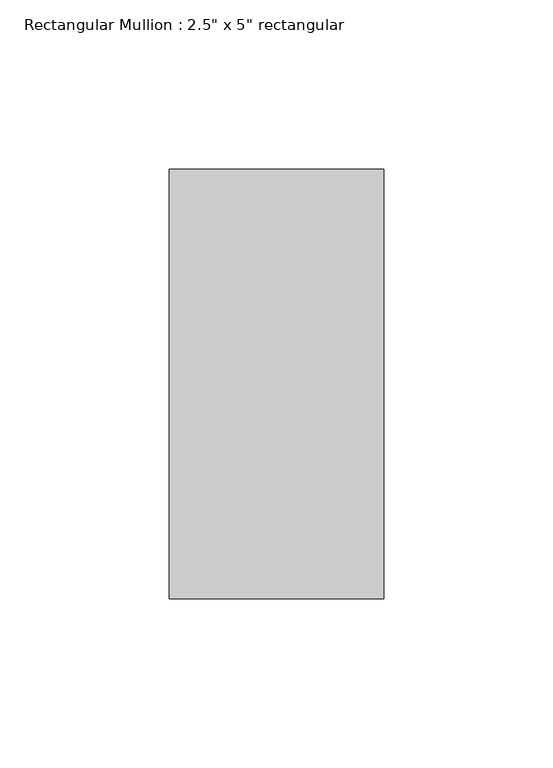
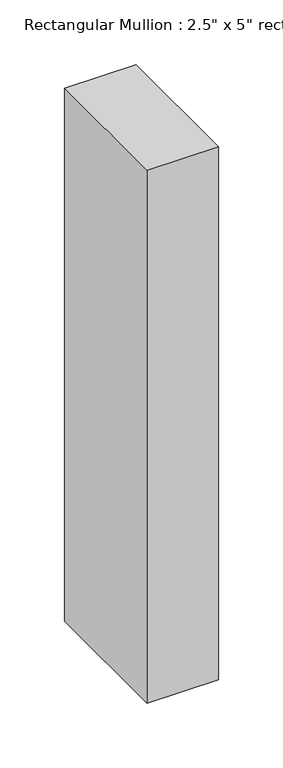
"""IFC4 building model written with IfcOpenShell, lengths in millimetres: member geometry."""

from ifc_helpers import new_model, si_unit, frame, origin, place, context, project, spatial, polyline, outline, extrude, source, transform, mapped, element, save


def member_45f9c1ec(model_context):
    return source(origin(), model_context, "Body", "SweptSolid", [
        extrude(outline(polyline([(0.0, 63.5), (0.0, -63.5), (-63.5, -63.5), (-63.5, 63.5), (0.0, 63.5)])), frame((0.0, 0.0, -501.65), z_axis=(0.0, 0.0, 1.0), x_axis=(1.0, 0.0, 0.0)), (0.0, 0.0, 1.0), 501.65),
    ])


if __name__ == "__main__":
    model = new_model("IFC4")
    model_context = context("Model", 3, world=origin())
    ifc_project = project(units=[si_unit("LENGTHUNIT", "METRE", prefix="MILLI")], contexts=[model_context])
    site = spatial("IfcSite", under=ifc_project)
    building = spatial("IfcBuilding", under=site)
    placement = place(None, origin())
    member_shape = member_45f9c1ec(model_context)
    element("IfcMember", 1, ObjectType="Rectangular Mullion : 2.5\" x 5\" rectangular", at=placement, inside=building, context=model_context, shape_type="MappedRepresentation", body=[
        mapped(member_shape, transform((0.0, 0.0, 0.0), x_axis=(1.0, 0.0, 0.0), y_axis=(0.0, 1.0, 0.0), z_axis=(0.0, 0.0, 1.0))),
    ])
    save(model, "model.ifc")

# Revit data of these elements
# Type "Rectangular Mullion : 2.5\" x 5\" rectangular"
#   built-in parameter 1007304 = 0.416667 (stored number, unit not read)
#   built-in parameter 1007301 = 0.104167 (stored number, unit not read)
#   built-in parameter 1007300 = 0.104167 (stored number, unit not read)
# Element 1 (IfcMember, "Rectangular Mullion : 2.5\" x 5\" rectangular")
#   Materials on its faces: "Aluminum"
# Materials
#   "Aluminum": class "Metal", colour RGB 247 247 247, transparency 0, Description = "Aluminum 6061", Cost = 0
